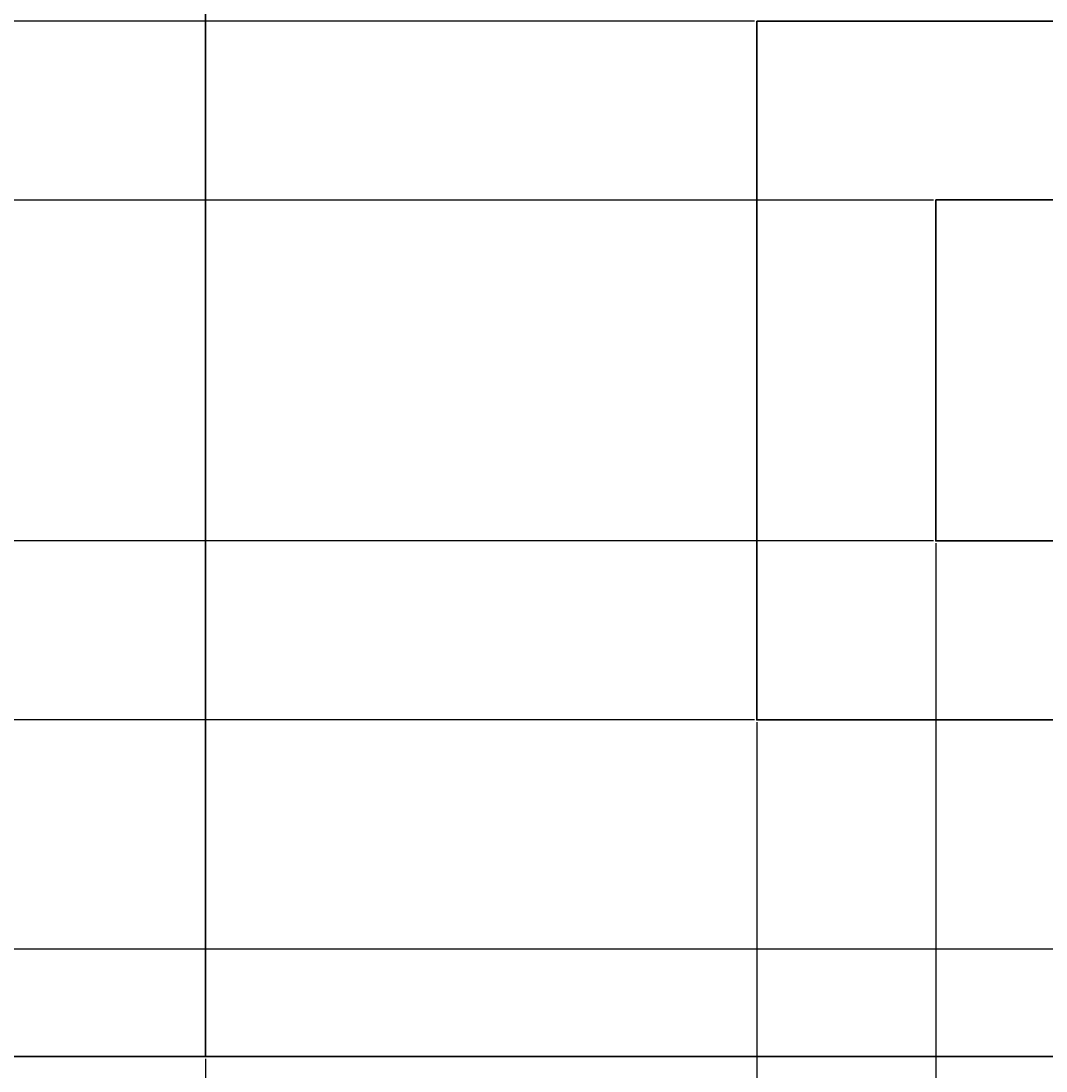
# Model space of a CAD drawing. Units: inches. Extents: x -6 to 289, y -8 to 323.
# Tile 4 of 107: x 19 to 48, y 7 to 36. Entities that reach past the tile are written whole.
import ezdxf

# ---------------------------------------------------------------- set-up
doc = ezdxf.new("R2010")
doc.units = ezdxf.units.IN
doc.header["$MEASUREMENT"] = 0
doc.layers.add('A-ANNO-DIMS', color=2, linetype='Continuous', lineweight=18)
doc.layers.add('A-ELEV', color=7, linetype='Continuous', lineweight=35)
doc.styles.get("Standard").update_dxf_attribs({"font": 'arial.ttf'})
doc.dimstyles.get("Standard").update_dxf_attribs({"dimtxt": 0.18, "dimasz": 0.18, "dimexe": 0.18, "dimexo": 0.0625, "dimgap": 0.09, "dimtad": 0, "dimtih": 1, "dimtoh": 1, "dimdec": 4, "dimzin": 0, "dimdsep": 46, "dimtxsty": 'Standard', "dimcen": 0.09, "dimadec": 0, "dimazin": 0, "dimtfac": 1, "dimtdec": 4, "dimtofl": 0, "dimtmove": 0, "dimatfit": 3, "dimfxl": 1, "dimtolj": 1, "dimtzin": 0, "dimarcsym": 0})

# ---------------------------------------------------------------- blocks, each defined once
blk = doc.blocks.new('*D16')
at = {"layer": 'A-ANNO-DIMS', "color": 0, "lineweight": -2, "transparency": 16777216}
for p, q in [((9.943, 68.37), (9.943, -8.391)), ((272.973, 68.37), (272.973, -8.391)), ((10.123, -8.211), (140.993, -8.211)), ((272.793, -8.211), (141.923, -8.211))]:
    blk.add_line(p, q, dxfattribs=at)
at = {"layer": 'A-ANNO-DIMS', "color": 0, "transparency": 16777216}
for points in [[(10.123, -8.181), (10.123, -8.241), (9.943, -8.211)], [(272.793, -8.181), (272.793, -8.241), (272.973, -8.211)]]:
    blk.add_solid(points, dxfattribs=at)
at = {"layer": 'Defpoints', "color": 0, "transparency": 16777216}
for p in [(9.943, 68.432), (272.973, 68.432), (272.973, -8.211)]:
    blk.add_point(p, dxfattribs=at)
at = {"layer": 'A-ANNO-DIMS', "color": 0, "transparency": 16777216, "insert": (141.458, -8.211), "char_height": 0.18, "attachment_point": 5}
blk.add_mtext('\\A1;263.03', dxfattribs=at)
blk = doc.blocks.new('*D17')
at = {"layer": 'A-ANNO-DIMS', "color": 0, "lineweight": -2, "transparency": 16777216}
for p, q in [((33.681, 70.243), (-5.737, 70.243)), ((-5.557, 70.063), (-5.557, 38.948)), ((-5.557, 7.469), (-5.557, 38.584)), ((11.907, 7.289), (-5.737, 7.289))]:
    blk.add_line(p, q, dxfattribs=at)
at = {"layer": 'A-ANNO-DIMS', "color": 0, "transparency": 16777216}
for points in [[(-5.587, 70.063), (-5.527, 70.063), (-5.557, 70.243)], [(-5.587, 7.469), (-5.527, 7.469), (-5.557, 7.289)]]:
    blk.add_solid(points, dxfattribs=at)
at = {"layer": 'Defpoints', "color": 0, "transparency": 16777216}
for p in [(-5.557, 70.243), (33.744, 70.243), (11.969, 7.289)]:
    blk.add_point(p, dxfattribs=at)
at = {"layer": 'A-ANNO-DIMS', "color": 0, "transparency": 16777216, "insert": (-5.557, 38.766), "char_height": 0.18, "attachment_point": 5}
blk.add_mtext('\\A1;62.95', dxfattribs=at)
blk = doc.blocks.new('*D50')
at = {"layer": 'A-ANNO-DIMS', "color": 0, "lineweight": -2, "transparency": 16777216}
for p, q in [((11.969, 7.226), (11.969, -8.391)), ((24.317, 7.226), (24.317, -8.391)), ((12.149, -8.211), (17.688, -8.211)), ((24.137, -8.211), (18.598, -8.211))]:
    blk.add_line(p, q, dxfattribs=at)
at = {"layer": 'A-ANNO-DIMS', "color": 0, "transparency": 16777216}
for points in [[(12.149, -8.181), (12.149, -8.241), (11.969, -8.211)], [(24.137, -8.181), (24.137, -8.241), (24.317, -8.211)]]:
    blk.add_solid(points, dxfattribs=at)
at = {"layer": 'Defpoints', "color": 0, "transparency": 16777216}
for p in [(11.969, 7.289), (24.317, 7.289), (24.317, -8.211)]:
    blk.add_point(p, dxfattribs=at)
at = {"layer": 'A-ANNO-DIMS', "color": 0, "transparency": 16777216, "insert": (18.143, -8.211), "char_height": 0.18, "attachment_point": 5}
blk.add_mtext('\\A1;12.348', dxfattribs=at)
blk = doc.blocks.new('*D51')
at = {"layer": 'A-ANNO-DIMS', "color": 0, "lineweight": -2, "transparency": 16777216}
for p, q in [((39.709, 16.629), (39.709, -8.391)), ((24.317, 7.226), (24.317, -8.391)), ((24.497, -8.211), (31.559, -8.211)), ((39.529, -8.211), (32.467, -8.211))]:
    blk.add_line(p, q, dxfattribs=at)
at = {"layer": 'A-ANNO-DIMS', "color": 0, "transparency": 16777216}
for points in [[(24.497, -8.181), (24.497, -8.241), (24.317, -8.211)], [(39.529, -8.181), (39.529, -8.241), (39.709, -8.211)]]:
    blk.add_solid(points, dxfattribs=at)
at = {"layer": 'Defpoints', "color": 0, "transparency": 16777216}
for p in [(39.709, 16.692), (24.317, 7.289), (39.709, -8.211)]:
    blk.add_point(p, dxfattribs=at)
at = {"layer": 'A-ANNO-DIMS', "color": 0, "transparency": 16777216, "insert": (32.013, -8.211), "char_height": 0.18, "attachment_point": 5}
blk.add_mtext('\\A1;15.392', dxfattribs=at)
blk = doc.blocks.new('*D52')
at = {"layer": 'A-ANNO-DIMS', "color": 0, "lineweight": -2, "transparency": 16777216}
for p, q in [((44.709, 21.629), (44.709, -8.391)), ((39.709, 16.629), (39.709, -8.391)), ((39.889, -8.211), (42.059, -8.211)), ((44.529, -8.211), (42.359, -8.211))]:
    blk.add_line(p, q, dxfattribs=at)
at = {"layer": 'A-ANNO-DIMS', "color": 0, "transparency": 16777216}
for points in [[(39.889, -8.181), (39.889, -8.241), (39.709, -8.211)], [(44.529, -8.181), (44.529, -8.241), (44.709, -8.211)]]:
    blk.add_solid(points, dxfattribs=at)
at = {"layer": 'Defpoints', "color": 0, "transparency": 16777216}
for p in [(44.709, 21.692), (39.709, 16.692), (44.709, -8.211)]:
    blk.add_point(p, dxfattribs=at)
at = {"layer": 'A-ANNO-DIMS', "color": 0, "transparency": 16777216, "insert": (42.209, -8.211), "char_height": 0.18, "attachment_point": 5}
blk.add_mtext('\\A1;5', dxfattribs=at)
blk = doc.blocks.new('*D53')
at = {"layer": 'A-ANNO-DIMS', "color": 0, "lineweight": -2, "transparency": 16777216}
for p, q in [((44.709, 21.629), (44.709, -8.391)), ((87.562, 21.629), (87.562, -8.391)), ((44.889, -8.211), (65.738, -8.211)), ((87.382, -8.211), (66.534, -8.211))]:
    blk.add_line(p, q, dxfattribs=at)
at = {"layer": 'A-ANNO-DIMS', "color": 0, "transparency": 16777216}
for points in [[(44.889, -8.181), (44.889, -8.241), (44.709, -8.211)], [(87.382, -8.181), (87.382, -8.241), (87.562, -8.211)]]:
    blk.add_solid(points, dxfattribs=at)
at = {"layer": 'Defpoints', "color": 0, "transparency": 16777216}
for p in [(44.709, 21.692), (87.562, 21.692), (87.562, -8.211)]:
    blk.add_point(p, dxfattribs=at)
at = {"layer": 'A-ANNO-DIMS', "color": 0, "transparency": 16777216, "insert": (66.136, -8.211), "char_height": 0.18, "attachment_point": 5}
blk.add_mtext('\\A1;42.85', dxfattribs=at)
blk = doc.blocks.new('*D59')
at = {"layer": 'A-ANNO-DIMS', "color": 0, "lineweight": -2, "transparency": 16777216}
for p, q in [((39.647, 16.692), (-5.737, 16.692)), ((-5.557, 16.512), (-5.557, 12.172)), ((-5.557, 7.469), (-5.557, 11.808)), ((11.907, 7.289), (-5.737, 7.289))]:
    blk.add_line(p, q, dxfattribs=at)
at = {"layer": 'A-ANNO-DIMS', "color": 0, "transparency": 16777216}
for points in [[(-5.587, 16.512), (-5.527, 16.512), (-5.557, 16.692)], [(-5.587, 7.469), (-5.527, 7.469), (-5.557, 7.289)]]:
    blk.add_solid(points, dxfattribs=at)
at = {"layer": 'Defpoints', "color": 0, "transparency": 16777216}
for p in [(-5.557, 16.692), (39.709, 16.692), (11.969, 7.289)]:
    blk.add_point(p, dxfattribs=at)
at = {"layer": 'A-ANNO-DIMS', "color": 0, "transparency": 16777216, "insert": (-5.557, 11.99), "char_height": 0.18, "attachment_point": 5}
blk.add_mtext('\\A1;9.403', dxfattribs=at)
blk = doc.blocks.new('*D60')
at = {"layer": 'A-ANNO-DIMS', "color": 0, "lineweight": -2, "transparency": 16777216}
for p, q in [((44.647, 21.692), (-5.737, 21.692)), ((-5.557, 21.512), (-5.557, 19.373)), ((-5.557, 16.872), (-5.557, 19.01)), ((39.647, 16.692), (-5.737, 16.692))]:
    blk.add_line(p, q, dxfattribs=at)
at = {"layer": 'A-ANNO-DIMS', "color": 0, "transparency": 16777216}
for points in [[(-5.587, 21.512), (-5.527, 21.512), (-5.557, 21.692)], [(-5.587, 16.872), (-5.527, 16.872), (-5.557, 16.692)]]:
    blk.add_solid(points, dxfattribs=at)
at = {"layer": 'Defpoints', "color": 0, "transparency": 16777216}
for p in [(-5.557, 21.692), (44.709, 21.692), (39.709, 16.692)]:
    blk.add_point(p, dxfattribs=at)
at = {"layer": 'A-ANNO-DIMS', "color": 0, "transparency": 16777216, "insert": (-5.557, 19.192), "char_height": 0.18, "attachment_point": 5}
blk.add_mtext('\\A1;5', dxfattribs=at)
blk = doc.blocks.new('*D61')
at = {"layer": 'A-ANNO-DIMS', "color": 0, "lineweight": -2, "transparency": 16777216}
for p, q in [((44.647, 31.213), (-5.737, 31.213)), ((-5.557, 31.033), (-5.557, 26.634)), ((-5.557, 21.872), (-5.557, 26.271)), ((44.647, 21.692), (-5.737, 21.692))]:
    blk.add_line(p, q, dxfattribs=at)
at = {"layer": 'A-ANNO-DIMS', "color": 0, "transparency": 16777216}
for points in [[(-5.587, 31.033), (-5.527, 31.033), (-5.557, 31.213)], [(-5.587, 21.872), (-5.527, 21.872), (-5.557, 21.692)]]:
    blk.add_solid(points, dxfattribs=at)
at = {"layer": 'Defpoints', "color": 0, "transparency": 16777216}
for p in [(-5.557, 31.213), (44.709, 31.213), (44.709, 21.692)]:
    blk.add_point(p, dxfattribs=at)
at = {"layer": 'A-ANNO-DIMS', "color": 0, "transparency": 16777216, "insert": (-5.557, 26.453), "char_height": 0.18, "attachment_point": 5}
blk.add_mtext('\\A1;9.522', dxfattribs=at)
blk = doc.blocks.new('*D62')
at = {"layer": 'A-ANNO-DIMS', "color": 0, "lineweight": -2, "transparency": 16777216}
for p, q in [((39.647, 36.213), (-5.737, 36.213)), ((-5.557, 36.033), (-5.557, 33.895)), ((-5.557, 31.393), (-5.557, 33.532)), ((44.647, 31.213), (-5.737, 31.213))]:
    blk.add_line(p, q, dxfattribs=at)
at = {"layer": 'A-ANNO-DIMS', "color": 0, "transparency": 16777216}
for points in [[(-5.587, 36.033), (-5.527, 36.033), (-5.557, 36.213)], [(-5.587, 31.393), (-5.527, 31.393), (-5.557, 31.213)]]:
    blk.add_solid(points, dxfattribs=at)
at = {"layer": 'Defpoints', "color": 0, "transparency": 16777216}
for p in [(-5.557, 36.213), (39.709, 36.213), (44.709, 31.213)]:
    blk.add_point(p, dxfattribs=at)
at = {"layer": 'A-ANNO-DIMS', "color": 0, "transparency": 16777216, "insert": (-5.557, 33.713), "char_height": 0.18, "attachment_point": 5}
blk.add_mtext('\\A1;5', dxfattribs=at)
blk = doc.blocks.new('*D83')
at = {"layer": 'A-ANNO-DIMS', "color": 0, "lineweight": -2, "transparency": 16777216}
for p, q in [((123.945, 10.289), (-5.737, 10.289)), ((-5.557, 10.109), (-5.557, 8.971)), ((-5.557, 7.469), (-5.557, 8.607)), ((120.945, 7.289), (-5.737, 7.289))]:
    blk.add_line(p, q, dxfattribs=at)
at = {"layer": 'A-ANNO-DIMS', "color": 0, "transparency": 16777216}
for points in [[(-5.587, 10.109), (-5.527, 10.109), (-5.557, 10.289)], [(-5.587, 7.469), (-5.527, 7.469), (-5.557, 7.289)]]:
    blk.add_solid(points, dxfattribs=at)
at = {"layer": 'Defpoints', "color": 0, "transparency": 16777216}
for p in [(-5.557, 10.289), (124.008, 10.289), (121.008, 7.289)]:
    blk.add_point(p, dxfattribs=at)
at = {"layer": 'A-ANNO-DIMS', "color": 0, "transparency": 16777216, "insert": (-5.557, 8.789), "char_height": 0.18, "attachment_point": 5}
blk.add_mtext('\\A1;3', dxfattribs=at)
blk = doc.blocks.new('*D84')
at = {"layer": 'A-ANNO-DIMS', "color": 0, "lineweight": -2, "transparency": 16777216}
for p, q in [((123.945, 48.085), (-5.737, 48.085)), ((-5.557, 47.905), (-5.557, 29.369)), ((-5.557, 10.469), (-5.557, 29.005)), ((123.945, 10.289), (-5.737, 10.289))]:
    blk.add_line(p, q, dxfattribs=at)
at = {"layer": 'A-ANNO-DIMS', "color": 0, "transparency": 16777216}
for points in [[(-5.587, 47.905), (-5.527, 47.905), (-5.557, 48.085)], [(-5.587, 10.469), (-5.527, 10.469), (-5.557, 10.289)]]:
    blk.add_solid(points, dxfattribs=at)
at = {"layer": 'Defpoints', "color": 0, "transparency": 16777216}
for p in [(-5.557, 48.085), (124.008, 48.085), (124.008, 10.289)]:
    blk.add_point(p, dxfattribs=at)
at = {"layer": 'A-ANNO-DIMS', "color": 0, "transparency": 16777216, "insert": (-5.557, 29.187), "char_height": 0.18, "attachment_point": 5}
blk.add_mtext('\\A1;37.8', dxfattribs=at)

msp = doc.modelspace()

# ---------------------------------------------------------------- linework, layer by layer
at = {"layer": 'A-ELEV'}
msp.add_line((19.1638, 7.2888), (271.1638, 7.2888), dxfattribs=at)
msp.add_lwpolyline([(11.9692, 66.2238), (11.9692, 7.2888), (24.317, 7.2888), (24.317, 66.2238)], dxfattribs=at)
for points in [[(24.317, 49.3604), (108.6602, 49.3604), (108.6602, 7.2888), (24.317, 7.2888)], [(39.709, 36.2133), (92.5623, 36.2133), (92.5623, 16.6917), (39.709, 16.6917)], [(44.709, 31.2133), (87.5623, 31.2133), (87.5623, 21.6917), (44.709, 21.6917)]]:
    msp.add_lwpolyline(points, close=True, dxfattribs=at)

# ---------------------------------------------------------------- dimensions: what is measured, and where the dimension line sits
at = {"layer": 'A-ANNO-DIMS'}
for base, p1, p2, override, picture, middle in [((-5.557, 70.2425), (11.9692, 7.2888), (33.7437, 70.2425), {"dimdec": 2, "dimlfac": 1, "dimrnd": 0, "dimzin": 0, "dimdsep": 46, "dimlunit": 2}, '*D17', (-5.557, 38.7657)), ((-5.557, 48.0851), (124.008, 10.2888), (124.008, 48.0851), {"dimdec": 1, "dimlfac": 1, "dimrnd": 0, "dimzin": 0, "dimdsep": 46, "dimlunit": 2}, '*D84', (-5.557, 29.187)), ((-5.557, 36.2133), (44.709, 31.2133), (39.709, 36.2133), {"dimdec": 0, "dimlfac": 1, "dimrnd": 0, "dimzin": 0, "dimdsep": 46, "dimlunit": 2}, '*D62', (-5.557, 33.7133)), ((-5.557, 31.2133), (44.709, 21.6917), (44.709, 31.2133), {"dimdec": 3, "dimlfac": 1, "dimrnd": 0, "dimzin": 0, "dimdsep": 46, "dimlunit": 2}, '*D61', (-5.557, 26.4525)), ((-5.557, 21.6917), (39.709, 16.6917), (44.709, 21.6917), {"dimdec": 0, "dimlfac": 1, "dimrnd": 0, "dimzin": 0, "dimdsep": 46, "dimlunit": 2}, '*D60', (-5.557, 19.1917)), ((-5.557, 16.6917), (11.9692, 7.2888), (39.709, 16.6917), {"dimdec": 3, "dimlfac": 1, "dimrnd": 0, "dimzin": 0, "dimdsep": 46, "dimlunit": 2}, '*D59', (-5.557, 11.9902)), ((-5.557, 10.2888), (121.008, 7.2888), (124.008, 10.2888), {"dimdec": 0, "dimlfac": 1, "dimrnd": 0, "dimzin": 0, "dimdsep": 46, "dimlunit": 2}, '*D83', (-5.557, 8.7888))]:
    dim = msp.add_linear_dim(base=base, p1=p1, p2=p2, angle=90, dimstyle='Standard', override=override, dxfattribs=at)
    dim.commit()
    dim.dimension.update_dxf_attribs({"geometry": picture, "text_midpoint": middle})
for base, p1, p2, override, picture, middle in [((272.9733, -8.2112), (9.943, 68.4322), (272.9733, 68.4322), {"dimdec": 2, "dimlfac": 1, "dimrnd": 0, "dimzin": 0, "dimdsep": 46, "dimlunit": 2}, '*D16', (141.4581, -8.2112)), ((44.709, -8.2112), (39.709, 16.6917), (44.709, 21.6917), {"dimdec": 0, "dimlfac": 1, "dimrnd": 0, "dimzin": 0, "dimdsep": 46, "dimlunit": 2}, '*D52', (42.209, -8.2112)), ((87.5623, -8.2112), (44.709, 21.6917), (87.5623, 21.6917), {"dimdec": 2, "dimlfac": 1, "dimrnd": 0, "dimzin": 0, "dimdsep": 46, "dimlunit": 2}, '*D53', (66.1357, -8.2112)), ((39.709, -8.2112), (24.317, 7.2888), (39.709, 16.6917), {"dimdec": 3, "dimlfac": 1, "dimrnd": 0, "dimzin": 0, "dimdsep": 46, "dimlunit": 2}, '*D51', (32.013, -8.2112)), ((24.317, -8.2112), (11.9692, 7.2888), (24.317, 7.2888), {"dimdec": 3, "dimlfac": 1, "dimrnd": 0, "dimzin": 0, "dimdsep": 46, "dimlunit": 2}, '*D50', (18.1431, -8.2112))]:
    dim = msp.add_linear_dim(base=base, p1=p1, p2=p2, dimstyle='Standard', override=override, dxfattribs=at)
    dim.commit()
    dim.dimension.update_dxf_attribs({"geometry": picture, "text_midpoint": middle})

doc.saveas('drawing.dxf')
